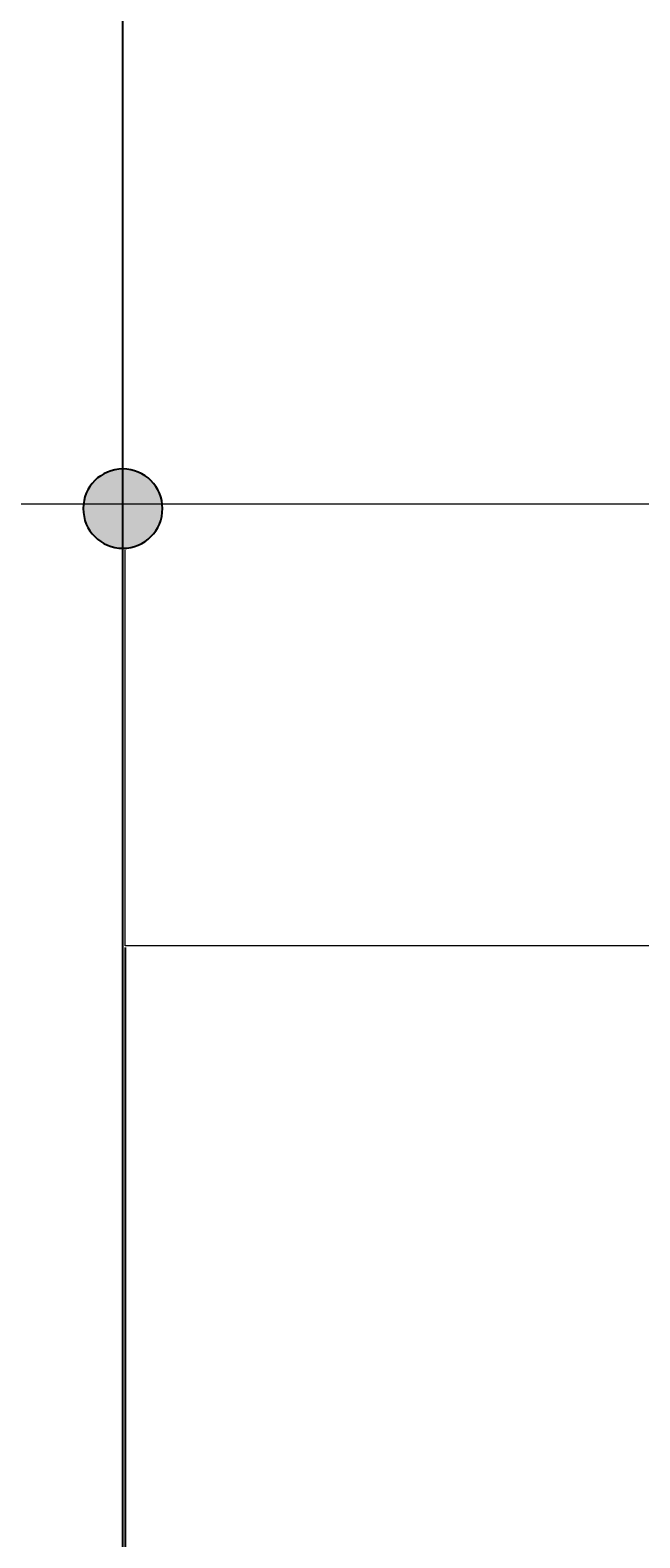
# Model space of a CAD drawing. Units: inches. Extents: x 738 to 1068, y 378 to 757.
# Tile 27 of 41: x 833 to 856, y 492 to 549. Entities that reach past the tile are written whole.
import ezdxf

# ---------------------------------------------------------------- set-up
doc = ezdxf.new("R2010")
doc.units = ezdxf.units.IN
doc.header["$MEASUREMENT"] = 0
for name, color, linetype, lineweight in [('A-ANNO-DIMS', 2, 'Continuous', 18), ('E-CONN', 7, 'Continuous', 25), ('E-CONN-PATT', 7, 'Continuous', 13), ('E-CTRL-WIRE', 7, 'Continuous', 18)]:
    doc.layers.add(name, color=color, linetype=linetype, lineweight=lineweight)
doc.styles.get("Standard").update_dxf_attribs({"font": 'arial.ttf'})
doc.dimstyles.get("Standard").update_dxf_attribs({"dimtxt": 0.18, "dimasz": 0.18, "dimexe": 0.18, "dimexo": 0.0625, "dimgap": 0.09, "dimtad": 0, "dimtih": 1, "dimtoh": 1, "dimdec": 4, "dimzin": 0, "dimdsep": 46, "dimtxsty": 'Standard', "dimcen": 0.09, "dimadec": 0, "dimazin": 0, "dimtfac": 1, "dimtdec": 4, "dimtofl": 0, "dimtmove": 0, "dimatfit": 3, "dimfxl": 1, "dimtolj": 1, "dimtzin": 0, "dimarcsym": 0})

# ---------------------------------------------------------------- blocks, each defined once
blk = doc.blocks.new('*D32')
at = {"layer": 'A-ANNO-DIMS', "color": 0, "lineweight": -2, "transparency": 16777216}
for p, q in [((809.38, 461.454), (809.38, 756.505)), ((809.56, 756.325), (822.41, 756.325)), ((836.052, 756.325), (823.202, 756.325)), ((836.232, 461.277), (836.232, 756.505))]:
    blk.add_line(p, q, dxfattribs=at)
at = {"layer": 'A-ANNO-DIMS', "color": 0, "transparency": 16777216}
for points in [[(809.56, 756.355), (809.56, 756.295), (809.38, 756.325)], [(836.052, 756.355), (836.052, 756.295), (836.232, 756.325)]]:
    blk.add_solid(points, dxfattribs=at)
at = {"layer": 'Defpoints', "color": 0, "transparency": 16777216}
for p in [(836.232, 756.325), (809.38, 461.392), (836.232, 461.214)]:
    blk.add_point(p, dxfattribs=at)
at = {"layer": 'A-ANNO-DIMS', "color": 0, "transparency": 16777216, "insert": (822.806, 756.325), "char_height": 0.18, "attachment_point": 5}
blk.add_mtext('\\A1;26.85', dxfattribs=at)
blk = doc.blocks.new('*D33')
at = {"layer": 'A-ANNO-DIMS', "color": 0, "lineweight": -2, "transparency": 16777216}
for p, q in [((836.324, 514.624), (836.324, 378.239)), ((907.171, 514.624), (907.171, 378.239)), ((836.504, 378.419), (871.354, 378.419)), ((906.991, 378.419), (872.141, 378.419))]:
    blk.add_line(p, q, dxfattribs=at)
at = {"layer": 'A-ANNO-DIMS', "color": 0, "transparency": 16777216}
for points in [[(836.504, 378.449), (836.504, 378.389), (836.324, 378.419)], [(906.991, 378.449), (906.991, 378.389), (907.171, 378.419)]]:
    blk.add_solid(points, dxfattribs=at)
at = {"layer": 'Defpoints', "color": 0, "transparency": 16777216}
for p in [(836.324, 514.687), (907.171, 514.687), (907.171, 378.419)]:
    blk.add_point(p, dxfattribs=at)
at = {"layer": 'A-ANNO-DIMS', "color": 0, "transparency": 16777216, "insert": (871.748, 378.419), "char_height": 0.18, "attachment_point": 5}
blk.add_mtext('\\A1;70.85', dxfattribs=at)
blk = doc.blocks.new('*D38')
at = {"layer": 'A-ANNO-DIMS', "color": 0, "lineweight": -2, "transparency": 16777216}
for p, q in [((781.485, 593.017), (781.485, 378.239)), ((887.04, 593.067), (887.04, 378.239)), ((781.665, 378.419), (833.807, 378.419)), ((886.86, 378.419), (834.718, 378.419))]:
    blk.add_line(p, q, dxfattribs=at)
at = {"layer": 'A-ANNO-DIMS', "color": 0, "transparency": 16777216}
for points in [[(781.665, 378.449), (781.665, 378.389), (781.485, 378.419)], [(886.86, 378.449), (886.86, 378.389), (887.04, 378.419)]]:
    blk.add_solid(points, dxfattribs=at)
at = {"layer": 'Defpoints', "color": 0, "transparency": 16777216}
for p in [(781.485, 593.08), (887.04, 593.13), (887.04, 378.419)]:
    blk.add_point(p, dxfattribs=at)
at = {"layer": 'A-ANNO-DIMS', "color": 0, "transparency": 16777216, "insert": (834.263, 378.419), "char_height": 0.18, "attachment_point": 5}
blk.add_mtext('\\A1;105.56', dxfattribs=at)

msp = doc.modelspace()

# ---------------------------------------------------------------- hatches: boundary and pattern name
at = {"layer": 'E-CONN-PATT'}
h = msp.add_hatch(color=256, dxfattribs=at)
h.dxf.hatch_style = 1
h.paths.add_polyline_path([(834.743, 531.4009), (837.7218, 531.4009, 0.8876841)])
h.paths.add_polyline_path([(837.7324, 531.2231, 0.0297234), (837.7218, 531.4009), (834.743, 531.4009, 0.0297234), (834.7324, 531.2231, 1)])
h.paths.add_polyline_path([(908.7522, 531.2231, 0.0297234), (908.7416, 531.4009), (905.7628, 531.4009, 0.0297234), (905.7522, 531.2231, 1)])
h.paths.add_polyline_path([(905.7628, 531.4009), (908.7416, 531.4009, 0.8876841)])

# ---------------------------------------------------------------- linework, layer by layer
at = {"layer": 'E-CONN'}
msp.add_lwpolyline([(834.7324, 531.2231, 1), (837.7324, 531.2231, 1)], format="xyb", close=True, dxfattribs=at)
at = {"layer": 'E-CTRL-WIRE'}
for p, q in [((809.3803, 531.4009), (865.0964, 531.4009)), ((836.3244, 514.6866), (836.3244, 529.6579)), ((866.3244, 514.6866), (836.3244, 514.6866))]:
    msp.add_line(p, q, dxfattribs=at)

# ---------------------------------------------------------------- dimensions: what is measured, and where the dimension line sits
at = {"layer": 'A-ANNO-DIMS'}
for base, p1, p2, picture, middle in [((836.2324, 756.3251), (809.3803, 461.3919), (836.2324, 461.214), '*D32', (822.8064, 756.3251)), ((887.0404, 378.4191), (781.4846, 593.0796), (887.0404, 593.1296), '*D38', (834.2625, 378.4191)), ((907.1708, 378.4191), (836.3244, 514.6866), (907.1708, 514.6866), '*D33', (871.7476, 378.4191))]:
    dim = msp.add_linear_dim(base=base, p1=p1, p2=p2, dimstyle='Standard', override={"dimdec": 2, "dimlfac": 1, "dimrnd": 0, "dimzin": 0, "dimdsep": 46, "dimlunit": 2}, dxfattribs=at)
    dim.commit()
    dim.dimension.update_dxf_attribs({"geometry": picture, "text_midpoint": middle})

doc.saveas('drawing.dxf')
